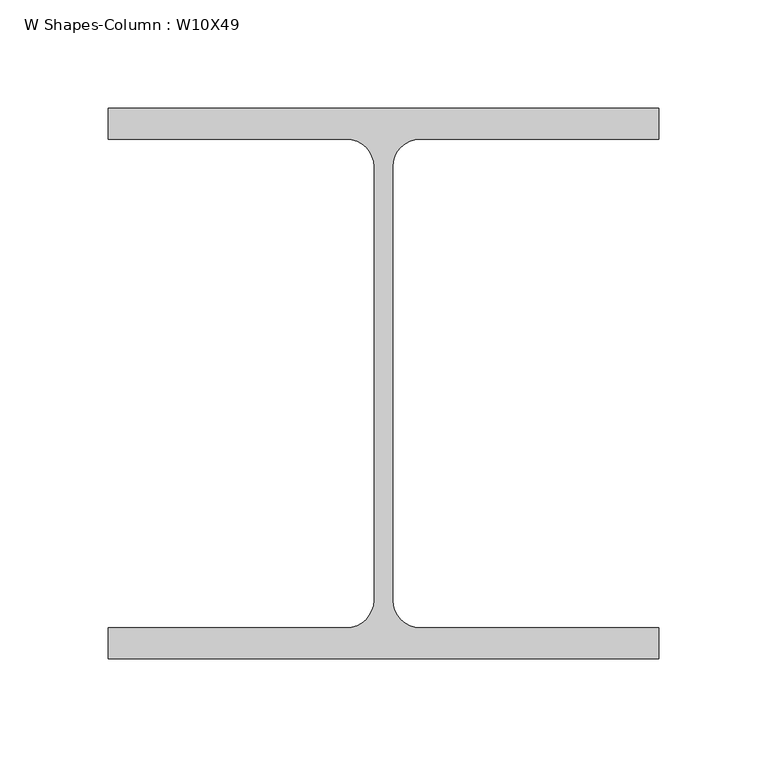
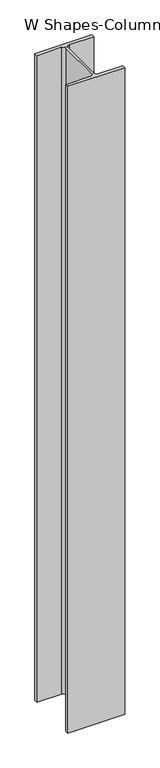
"""IFC4 building model written with IfcOpenShell, lengths in millimetres: column geometry, W Shapes-Column : W10X49."""

from ifc_helpers import new_model, si_unit, point, frame, frame_2d, origin, place, context, project, spatial, polyline, circle_curve, trimmed, segment, composite_curve, outline, extrude, source, transform, mapped, element, save


def w_shapes_column_w10x49_51893fb5(model_context):
    return source(origin(), model_context, "Body", "SweptSolid", [
        extrude(outline(composite_curve([segment(polyline([(127.0, 127.0), (127.0, 112.776), (17.018, 112.776)]), True, "CONTINUOUS"), segment(trimmed(circle_curve(frame_2d((17.018, 100.076)), 12.7), [point((17.018, 112.776))], [point((4.318, 100.076))], True, "CARTESIAN"), True, "CONTINUOUS"), segment(polyline([(4.318, 100.076), (4.318, -100.076)]), True, "CONTINUOUS"), segment(trimmed(circle_curve(frame_2d((17.018, -100.076)), 12.7), [point((4.318, -100.076))], [point((17.018, -112.776))], True, "CARTESIAN"), True, "CONTINUOUS"), segment(polyline([(17.018, -112.776), (127.0, -112.776), (127.0, -127.0), (-127.0, -127.0), (-127.0, -112.776), (-17.018, -112.776)]), True, "CONTINUOUS"), segment(trimmed(circle_curve(frame_2d((-17.018, -100.076)), 12.7), [point((-17.018, -112.776))], [point((-4.318, -100.076))], True, "CARTESIAN"), True, "CONTINUOUS"), segment(polyline([(-4.318, -100.076), (-4.318, 100.076)]), True, "CONTINUOUS"), segment(trimmed(circle_curve(frame_2d((-17.018, 100.076)), 12.7), [point((-4.318, 100.076))], [point((-17.018, 112.776))], True, "CARTESIAN"), True, "CONTINUOUS"), segment(polyline([(-17.018, 112.776), (-127.0, 112.776), (-127.0, 127.0), (127.0, 127.0)]), True, "CONTINUOUS")], self_intersect=False)), frame((0.0, 0.0, 12192.0), z_axis=(0.0, 0.0, 1.0), x_axis=(1.0, 0.0, 0.0)), (0.0, 0.0, 1.0), 3048.0),
    ])


if __name__ == "__main__":
    model = new_model("IFC4")
    model_context = context("Model", 3, world=origin())
    ifc_project = project(units=[si_unit("LENGTHUNIT", "METRE", prefix="MILLI")], contexts=[model_context])
    site = spatial("IfcSite", under=ifc_project)
    building = spatial("IfcBuilding", under=site)
    placement = place(None, origin())
    w_shapes_column_w10x49_shape = w_shapes_column_w10x49_51893fb5(model_context)
    element("IfcColumn", 1, ObjectType="W Shapes-Column : W10X49", at=placement, inside=building, context=model_context, shape_type="MappedRepresentation", body=[
        mapped(w_shapes_column_w10x49_shape, transform((0.0, 0.0, 0.0), x_axis=(1.0, 0.0, 0.0), y_axis=(0.0, 1.0, 0.0), z_axis=(0.0, 0.0, 1.0))),
    ])
    save(model, "model.ifc")

# Revit data of these elements
# Type "W Shapes-Column : W10X49"
#   Section Name Key = "W10x49"
#   Assembly Code = "B10"
#   Width = 10.000"
#   Web Thickness = 0.340"
#   Web Fillet = 0.500"
#   Warping Constant = 2070.00 in⁶
#   Torsional Moment of Inertia = 1.39 in⁴
#   Section Area = 14.40 in²
#   Plastic Modulus weak axis = 28.30 in³
#   Plastic Modulus strong axis = 60.40 in³
#   Perimeter = 58.50 ft²/ft
#   Nominal Weight = 49.00 lbf/ft
#   Moment of Inertia weak axis = 93.40 in⁴
#   Moment of Inertia strong axis = 272.00 in⁴
#   Height = 10.000"
#   Flange Thickness = 0.560"
#   Elastic Modulus weak axis = 18.70 in³
#   Elastic Modulus strong axis = 54.60 in³
#   Centroid Vertical = 5.000"
#   Centroid Horizontal = 5.000"
#   Bolt Spacing = 0' - 5 1/2"
#   Structural Material [instance default] = Steel ASTM A992
#   Principal Axes Angle = 0
# Element 1 (IfcColumn, "W Shapes-Column : W10X49")
#   Materials on its faces: "Steel ASTM A992"
# Materials
#   "Steel ASTM A992": class "Metal", colour RGB 199 199 199, transparency 0, Description = "Structural steel 50ksi", Cost = 0
